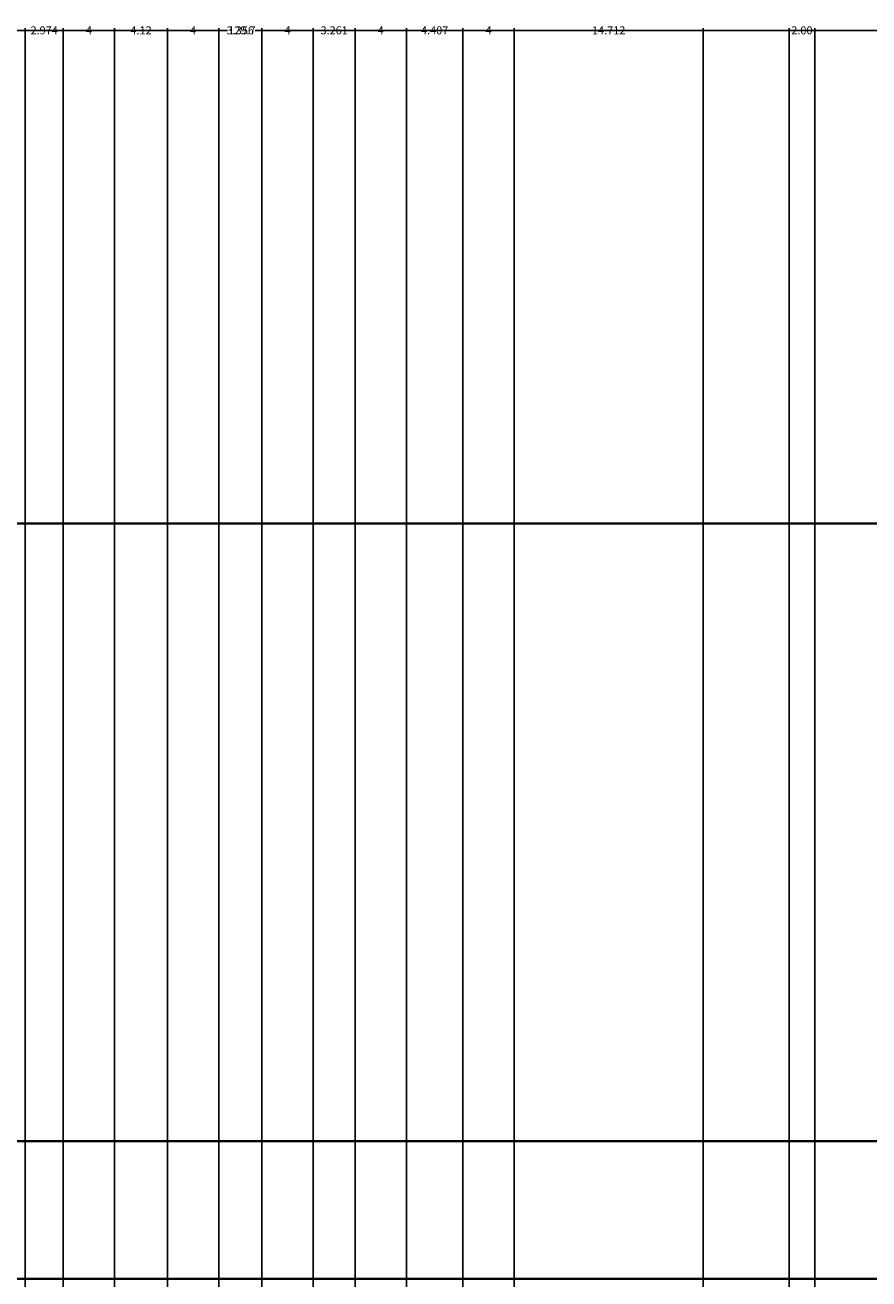
# Model space of a CAD drawing. Units: inches. Extents: x -13 to 809, y 112 to 656.
# Tile 39 of 55: x 389 to 455, y 559 to 656. Entities that reach past the tile are written whole.
import ezdxf

# ---------------------------------------------------------------- set-up
doc = ezdxf.new("R2010")
doc.units = ezdxf.units.IN
doc.header["$MEASUREMENT"] = 0
doc.layers.add('A-ANNO-DIMS', color=2, linetype='Continuous', lineweight=18)
doc.layers.add('A-ELEV', color=7, linetype='Continuous', lineweight=35)
doc.styles.get("Standard").update_dxf_attribs({"font": 'arial.ttf'})
doc.dimstyles.get("Standard").update_dxf_attribs({"dimtxt": 0.625, "dimasz": 0.18, "dimexe": 0.18, "dimexo": 0.0625, "dimgap": 0.09, "dimtad": 0, "dimtih": 1, "dimtoh": 1, "dimdec": 4, "dimzin": 0, "dimdsep": 46, "dimlunit": 4, "dimtxsty": 'Standard', "dimcen": 0.09, "dimadec": 0, "dimazin": 0, "dimtfac": 1, "dimtdec": 4, "dimtofl": 0, "dimtmove": 0, "dimatfit": 3, "dimfxl": 1, "dimtolj": 1, "dimtzin": 0, "dimarcsym": 0})

# ---------------------------------------------------------------- blocks, each defined once
blk = doc.blocks.new('*D26')
at = {"layer": 'A-ANNO-DIMS', "color": 0, "lineweight": -2, "transparency": 16777216}
for p, q in [((341.407, 524.343), (341.407, 655.963)), ((341.587, 655.783), (405.138, 655.783)), ((470.92, 655.783), (407.369, 655.783)), ((471.1, 470.939), (471.1, 655.963))]:
    blk.add_line(p, q, dxfattribs=at)
at = {"layer": 'A-ANNO-DIMS', "color": 0, "transparency": 16777216}
for points in [[(341.587, 655.813), (341.587, 655.753), (341.407, 655.783)], [(470.92, 655.813), (470.92, 655.753), (471.1, 655.783)]]:
    blk.add_solid(points, dxfattribs=at)
at = {"layer": 'Defpoints', "color": 0, "transparency": 16777216}
for p in [(471.1, 655.783), (341.407, 524.281), (471.1, 470.877)]:
    blk.add_point(p, dxfattribs=at)
at = {"layer": 'A-ANNO-DIMS', "color": 0, "transparency": 16777216, "insert": (406.253, 655.783), "char_height": 0.625, "attachment_point": 5}
blk.add_mtext('\\A1;129.7', dxfattribs=at)
blk = doc.blocks.new('*D63')
at = {"layer": 'A-ANNO-DIMS', "color": 0, "lineweight": -2, "transparency": 16777216}
for p, q in [((389.354, 524.343), (389.354, 655.963)), ((389.534, 655.783), (389.692, 655.783)), ((392.148, 655.783), (391.989, 655.783)), ((392.328, 524.343), (392.328, 655.963))]:
    blk.add_line(p, q, dxfattribs=at)
at = {"layer": 'A-ANNO-DIMS', "color": 0, "transparency": 16777216}
for points in [[(389.534, 655.813), (389.534, 655.753), (389.354, 655.783)], [(392.148, 655.813), (392.148, 655.753), (392.328, 655.783)]]:
    blk.add_solid(points, dxfattribs=at)
at = {"layer": 'Defpoints', "color": 0, "transparency": 16777216}
for p in [(392.328, 655.783), (389.354, 524.281), (392.328, 524.281)]:
    blk.add_point(p, dxfattribs=at)
at = {"layer": 'A-ANNO-DIMS', "color": 0, "transparency": 16777216, "insert": (390.841, 655.783), "char_height": 0.625, "attachment_point": 5}
blk.add_mtext('\\A1;2.974', dxfattribs=at)
blk = doc.blocks.new('*D64')
at = {"layer": 'A-ANNO-DIMS', "color": 0, "lineweight": -2, "transparency": 16777216}
for p, q in [((392.328, 524.343), (392.328, 655.963)), ((392.508, 655.783), (394.022, 655.783)), ((396.148, 655.783), (394.634, 655.783)), ((396.328, 524.343), (396.328, 655.963))]:
    blk.add_line(p, q, dxfattribs=at)
at = {"layer": 'A-ANNO-DIMS', "color": 0, "transparency": 16777216}
for points in [[(392.508, 655.813), (392.508, 655.753), (392.328, 655.783)], [(396.148, 655.813), (396.148, 655.753), (396.328, 655.783)]]:
    blk.add_solid(points, dxfattribs=at)
at = {"layer": 'Defpoints', "color": 0, "transparency": 16777216}
for p in [(396.328, 655.783), (392.328, 524.281), (396.328, 524.281)]:
    blk.add_point(p, dxfattribs=at)
at = {"layer": 'A-ANNO-DIMS', "color": 0, "transparency": 16777216, "insert": (394.328, 655.783), "char_height": 0.625, "attachment_point": 5}
blk.add_mtext('\\A1;4', dxfattribs=at)
blk = doc.blocks.new('*D65')
at = {"layer": 'A-ANNO-DIMS', "color": 0, "lineweight": -2, "transparency": 16777216}
for p, q in [((396.328, 524.343), (396.328, 655.963)), ((396.508, 655.783), (397.477, 655.783)), ((400.268, 655.783), (399.299, 655.783)), ((400.448, 524.343), (400.448, 655.963))]:
    blk.add_line(p, q, dxfattribs=at)
at = {"layer": 'A-ANNO-DIMS', "color": 0, "transparency": 16777216}
for points in [[(396.508, 655.813), (396.508, 655.753), (396.328, 655.783)], [(400.268, 655.813), (400.268, 655.753), (400.448, 655.783)]]:
    blk.add_solid(points, dxfattribs=at)
at = {"layer": 'Defpoints', "color": 0, "transparency": 16777216}
for p in [(400.448, 655.783), (396.328, 524.281), (400.448, 524.281)]:
    blk.add_point(p, dxfattribs=at)
at = {"layer": 'A-ANNO-DIMS', "color": 0, "transparency": 16777216, "insert": (398.388, 655.783), "char_height": 0.625, "attachment_point": 5}
blk.add_mtext('\\A1;4.12', dxfattribs=at)
blk = doc.blocks.new('*D66')
at = {"layer": 'A-ANNO-DIMS', "color": 0, "lineweight": -2, "transparency": 16777216}
for p, q in [((400.448, 524.343), (400.448, 655.963)), ((400.628, 655.783), (402.142, 655.783)), ((404.268, 655.783), (402.754, 655.783)), ((404.448, 524.343), (404.448, 655.963))]:
    blk.add_line(p, q, dxfattribs=at)
at = {"layer": 'A-ANNO-DIMS', "color": 0, "transparency": 16777216}
for points in [[(400.628, 655.813), (400.628, 655.753), (400.448, 655.783)], [(404.268, 655.813), (404.268, 655.753), (404.448, 655.783)]]:
    blk.add_solid(points, dxfattribs=at)
at = {"layer": 'Defpoints', "color": 0, "transparency": 16777216}
for p in [(404.448, 655.783), (400.448, 524.281), (404.448, 524.281)]:
    blk.add_point(p, dxfattribs=at)
at = {"layer": 'A-ANNO-DIMS', "color": 0, "transparency": 16777216, "insert": (402.448, 655.783), "char_height": 0.625, "attachment_point": 5}
blk.add_mtext('\\A1;4', dxfattribs=at)
blk = doc.blocks.new('*D67')
at = {"layer": 'A-ANNO-DIMS', "color": 0, "lineweight": -2, "transparency": 16777216}
for p, q in [((404.448, 524.343), (404.448, 655.963)), ((404.628, 655.783), (404.982, 655.783)), ((407.625, 655.783), (407.271, 655.783)), ((407.805, 524.343), (407.805, 655.963))]:
    blk.add_line(p, q, dxfattribs=at)
at = {"layer": 'A-ANNO-DIMS', "color": 0, "transparency": 16777216}
for points in [[(404.628, 655.813), (404.628, 655.753), (404.448, 655.783)], [(407.625, 655.813), (407.625, 655.753), (407.805, 655.783)]]:
    blk.add_solid(points, dxfattribs=at)
at = {"layer": 'Defpoints', "color": 0, "transparency": 16777216}
for p in [(407.805, 655.783), (404.448, 524.281), (407.805, 524.281)]:
    blk.add_point(p, dxfattribs=at)
at = {"layer": 'A-ANNO-DIMS', "color": 0, "transparency": 16777216, "insert": (406.126, 655.783), "char_height": 0.625, "attachment_point": 5}
blk.add_mtext('\\A1;3.356', dxfattribs=at)
blk = doc.blocks.new('*D68')
at = {"layer": 'A-ANNO-DIMS', "color": 0, "lineweight": -2, "transparency": 16777216}
for p, q in [((407.805, 524.343), (407.805, 655.963)), ((407.985, 655.783), (409.498, 655.783)), ((411.625, 655.783), (410.111, 655.783)), ((411.805, 524.343), (411.805, 655.963))]:
    blk.add_line(p, q, dxfattribs=at)
at = {"layer": 'A-ANNO-DIMS', "color": 0, "transparency": 16777216}
for points in [[(407.985, 655.813), (407.985, 655.753), (407.805, 655.783)], [(411.625, 655.813), (411.625, 655.753), (411.805, 655.783)]]:
    blk.add_solid(points, dxfattribs=at)
at = {"layer": 'Defpoints', "color": 0, "transparency": 16777216}
for p in [(411.805, 655.783), (407.805, 524.281), (411.805, 524.281)]:
    blk.add_point(p, dxfattribs=at)
at = {"layer": 'A-ANNO-DIMS', "color": 0, "transparency": 16777216, "insert": (409.805, 655.783), "char_height": 0.625, "attachment_point": 5}
blk.add_mtext('\\A1;4', dxfattribs=at)
blk = doc.blocks.new('*D69')
at = {"layer": 'A-ANNO-DIMS', "color": 0, "lineweight": -2, "transparency": 16777216}
for p, q in [((411.805, 524.343), (411.805, 655.963)), ((411.985, 655.783), (412.351, 655.783)), ((414.885, 655.783), (414.519, 655.783)), ((415.065, 524.343), (415.065, 655.963))]:
    blk.add_line(p, q, dxfattribs=at)
at = {"layer": 'A-ANNO-DIMS', "color": 0, "transparency": 16777216}
for points in [[(411.985, 655.813), (411.985, 655.753), (411.805, 655.783)], [(414.885, 655.813), (414.885, 655.753), (415.065, 655.783)]]:
    blk.add_solid(points, dxfattribs=at)
at = {"layer": 'Defpoints', "color": 0, "transparency": 16777216}
for p in [(415.065, 655.783), (411.805, 524.281), (415.065, 524.281)]:
    blk.add_point(p, dxfattribs=at)
at = {"layer": 'A-ANNO-DIMS', "color": 0, "transparency": 16777216, "insert": (413.435, 655.783), "char_height": 0.625, "attachment_point": 5}
blk.add_mtext('\\A1;3.261', dxfattribs=at)
blk = doc.blocks.new('*D70')
at = {"layer": 'A-ANNO-DIMS', "color": 0, "lineweight": -2, "transparency": 16777216}
for p, q in [((415.065, 524.343), (415.065, 655.963)), ((415.245, 655.783), (416.759, 655.783)), ((418.885, 655.783), (417.371, 655.783)), ((419.065, 524.343), (419.065, 655.963))]:
    blk.add_line(p, q, dxfattribs=at)
at = {"layer": 'A-ANNO-DIMS', "color": 0, "transparency": 16777216}
for points in [[(415.245, 655.813), (415.245, 655.753), (415.065, 655.783)], [(418.885, 655.813), (418.885, 655.753), (419.065, 655.783)]]:
    blk.add_solid(points, dxfattribs=at)
at = {"layer": 'Defpoints', "color": 0, "transparency": 16777216}
for p in [(419.065, 655.783), (415.065, 524.281), (419.065, 524.281)]:
    blk.add_point(p, dxfattribs=at)
at = {"layer": 'A-ANNO-DIMS', "color": 0, "transparency": 16777216, "insert": (417.065, 655.783), "char_height": 0.625, "attachment_point": 5}
blk.add_mtext('\\A1;4', dxfattribs=at)
blk = doc.blocks.new('*D71')
at = {"layer": 'A-ANNO-DIMS', "color": 0, "lineweight": -2, "transparency": 16777216}
for p, q in [((419.065, 524.343), (419.065, 655.963)), ((419.245, 655.783), (420.112, 655.783)), ((423.292, 655.783), (422.426, 655.783)), ((423.472, 524.343), (423.472, 655.963))]:
    blk.add_line(p, q, dxfattribs=at)
at = {"layer": 'A-ANNO-DIMS', "color": 0, "transparency": 16777216}
for points in [[(419.245, 655.813), (419.245, 655.753), (419.065, 655.783)], [(423.292, 655.813), (423.292, 655.753), (423.472, 655.783)]]:
    blk.add_solid(points, dxfattribs=at)
at = {"layer": 'Defpoints', "color": 0, "transparency": 16777216}
for p in [(423.472, 655.783), (419.065, 524.281), (423.472, 524.281)]:
    blk.add_point(p, dxfattribs=at)
at = {"layer": 'A-ANNO-DIMS', "color": 0, "transparency": 16777216, "insert": (421.269, 655.783), "char_height": 0.625, "attachment_point": 5}
blk.add_mtext('\\A1;4.407', dxfattribs=at)
blk = doc.blocks.new('*D72')
at = {"layer": 'A-ANNO-DIMS', "color": 0, "lineweight": -2, "transparency": 16777216}
for p, q in [((423.472, 524.343), (423.472, 655.963)), ((423.652, 655.783), (425.166, 655.783)), ((427.292, 655.783), (425.779, 655.783)), ((427.472, 524.343), (427.472, 655.963))]:
    blk.add_line(p, q, dxfattribs=at)
at = {"layer": 'A-ANNO-DIMS', "color": 0, "transparency": 16777216}
for points in [[(423.652, 655.813), (423.652, 655.753), (423.472, 655.783)], [(427.292, 655.813), (427.292, 655.753), (427.472, 655.783)]]:
    blk.add_solid(points, dxfattribs=at)
at = {"layer": 'Defpoints', "color": 0, "transparency": 16777216}
for p in [(427.472, 655.783), (423.472, 524.281), (427.472, 524.281)]:
    blk.add_point(p, dxfattribs=at)
at = {"layer": 'A-ANNO-DIMS', "color": 0, "transparency": 16777216, "insert": (425.472, 655.783), "char_height": 0.625, "attachment_point": 5}
blk.add_mtext('\\A1;4', dxfattribs=at)
blk = doc.blocks.new('*D73')
at = {"layer": 'A-ANNO-DIMS', "color": 0, "lineweight": -2, "transparency": 16777216}
for p, q in [((427.472, 524.343), (427.472, 655.963)), ((427.652, 655.783), (433.474, 655.783)), ((442.004, 655.783), (436.183, 655.783)), ((442.184, 524.343), (442.184, 655.963))]:
    blk.add_line(p, q, dxfattribs=at)
at = {"layer": 'A-ANNO-DIMS', "color": 0, "transparency": 16777216}
for points in [[(427.652, 655.813), (427.652, 655.753), (427.472, 655.783)], [(442.004, 655.813), (442.004, 655.753), (442.184, 655.783)]]:
    blk.add_solid(points, dxfattribs=at)
at = {"layer": 'Defpoints', "color": 0, "transparency": 16777216}
for p in [(442.184, 655.783), (427.472, 524.281), (442.184, 524.281)]:
    blk.add_point(p, dxfattribs=at)
at = {"layer": 'A-ANNO-DIMS', "color": 0, "transparency": 16777216, "insert": (434.828, 655.783), "char_height": 0.625, "attachment_point": 5}
blk.add_mtext('\\A1;14.712', dxfattribs=at)
blk = doc.blocks.new('*D133')
at = {"layer": 'A-ANNO-DIMS', "color": 0, "lineweight": -2, "transparency": 16777216}
for p, q in [((448.701738, 655.782835), (448.521738, 655.782835)), ((448.881738, 207.535185), (448.881738, 655.962835)), ((450.881738, 207.527657), (450.881738, 655.962835)), ((451.061738, 655.782835), (451.241738, 655.782835))]:
    blk.add_line(p, q, dxfattribs=at)
at = {"layer": 'A-ANNO-DIMS', "color": 0, "transparency": 16777216}
for points in [[(448.701738, 655.812835), (448.701738, 655.752835), (448.881738, 655.782835)], [(451.061738, 655.812835), (451.061738, 655.752835), (450.881738, 655.782835)]]:
    blk.add_solid(points, dxfattribs=at)
at = {"layer": 'Defpoints', "color": 0, "transparency": 16777216}
for p in [(450.881738, 655.782835), (448.881738, 207.472685), (450.881738, 207.465157)]:
    blk.add_point(p, dxfattribs=at)
at = {"layer": 'A-ANNO-DIMS', "color": 0, "transparency": 16777216, "insert": (449.881738, 655.782835), "char_height": 0.625, "attachment_point": 5}
blk.add_mtext('\\A1;2.00', dxfattribs=at)

msp = doc.modelspace()

# ---------------------------------------------------------------- linework, layer by layer
at = {"layer": 'A-ELEV'}
for p, q in [((311.6991, 617.3708), (621.008, 617.3708)), ((292.923, 569.2414), (644.6221, 569.2414)), ((341.4072, 558.5199), (591.008, 558.5199))]:
    msp.add_line(p, q, dxfattribs=at)

# ---------------------------------------------------------------- dimensions: what is measured, and where the dimension line sits
at = {"layer": 'A-ANNO-DIMS'}
for base, p1, p2, override, picture, middle in [((471.0998, 655.7828), (341.4072, 524.281), (471.0998, 470.8765), {"dimdec": 1, "dimlfac": 1, "dimrnd": 0, "dimzin": 0, "dimdsep": 46, "dimlunit": 2}, '*D26', (406.2535, 655.7828)), ((392.3277, 655.7828), (389.3536, 524.281), (392.3277, 524.281), {"dimdec": 3, "dimlfac": 1, "dimrnd": 0, "dimzin": 0, "dimdsep": 46, "dimlunit": 2}, '*D63', (390.8407, 655.7828)), ((396.3277, 655.7828), (392.3277, 524.281), (396.3277, 524.281), {"dimdec": 0, "dimlfac": 1, "dimrnd": 0, "dimzin": 0, "dimdsep": 46, "dimlunit": 2}, '*D64', (394.3277, 655.7828)), ((400.4483, 655.7828), (396.3277, 524.281), (400.4483, 524.281), {"dimdec": 2, "dimlfac": 1, "dimrnd": 0, "dimzin": 0, "dimdsep": 46, "dimlunit": 2}, '*D65', (398.388, 655.7828)), ((404.4483, 655.7828), (400.4483, 524.281), (404.4483, 524.281), {"dimdec": 0, "dimlfac": 1, "dimrnd": 0, "dimzin": 0, "dimdsep": 46, "dimlunit": 2}, '*D66', (402.4483, 655.7828)), ((407.8046, 655.7828), (404.4483, 524.281), (407.8046, 524.281), {"dimdec": 3, "dimlfac": 1, "dimrnd": 0, "dimzin": 0, "dimdsep": 46, "dimlunit": 2}, '*D67', (406.1264, 655.7828)), ((411.8046, 655.7828), (407.8046, 524.281), (411.8046, 524.281), {"dimdec": 0, "dimlfac": 1, "dimrnd": 0, "dimzin": 0, "dimdsep": 46, "dimlunit": 2}, '*D68', (409.8046, 655.7828)), ((415.0653, 655.7828), (411.8046, 524.281), (415.0653, 524.281), {"dimdec": 3, "dimlfac": 1, "dimrnd": 0, "dimzin": 0, "dimdsep": 46, "dimlunit": 2}, '*D69', (413.4349, 655.7828)), ((419.0653, 655.7828), (415.0653, 524.281), (419.0653, 524.281), {"dimdec": 0, "dimlfac": 1, "dimrnd": 0, "dimzin": 0, "dimdsep": 46, "dimlunit": 2}, '*D70', (417.0653, 655.7828)), ((423.4725, 655.7828), (419.0653, 524.281), (423.4725, 524.281), {"dimdec": 3, "dimlfac": 1, "dimrnd": 0, "dimzin": 0, "dimdsep": 46, "dimlunit": 2}, '*D71', (421.2689, 655.7828)), ((427.4725, 655.7828), (423.4725, 524.281), (427.4725, 524.281), {"dimdec": 0, "dimlfac": 1, "dimrnd": 0, "dimzin": 0, "dimdsep": 46, "dimlunit": 2}, '*D72', (425.4725, 655.7828)), ((442.1845, 655.7828), (427.4725, 524.281), (442.1845, 524.281), {"dimdec": 3, "dimlfac": 1, "dimrnd": 0, "dimzin": 0, "dimdsep": 46, "dimlunit": 2}, '*D73', (434.8285, 655.7828)), ((450.8817, 655.7828), (448.8817, 207.4727), (450.8817, 207.4652), {"dimdec": 2, "dimlfac": 1, "dimrnd": 0, "dimzin": 0, "dimdsep": 46, "dimlunit": 2}, '*D133', (449.8817, 655.7828))]:
    dim = msp.add_linear_dim(base=base, p1=p1, p2=p2, dimstyle='Standard', override=override, dxfattribs=at)
    dim.commit()
    dim.dimension.update_dxf_attribs({"geometry": picture, "text_midpoint": middle})

doc.saveas('drawing.dxf')
